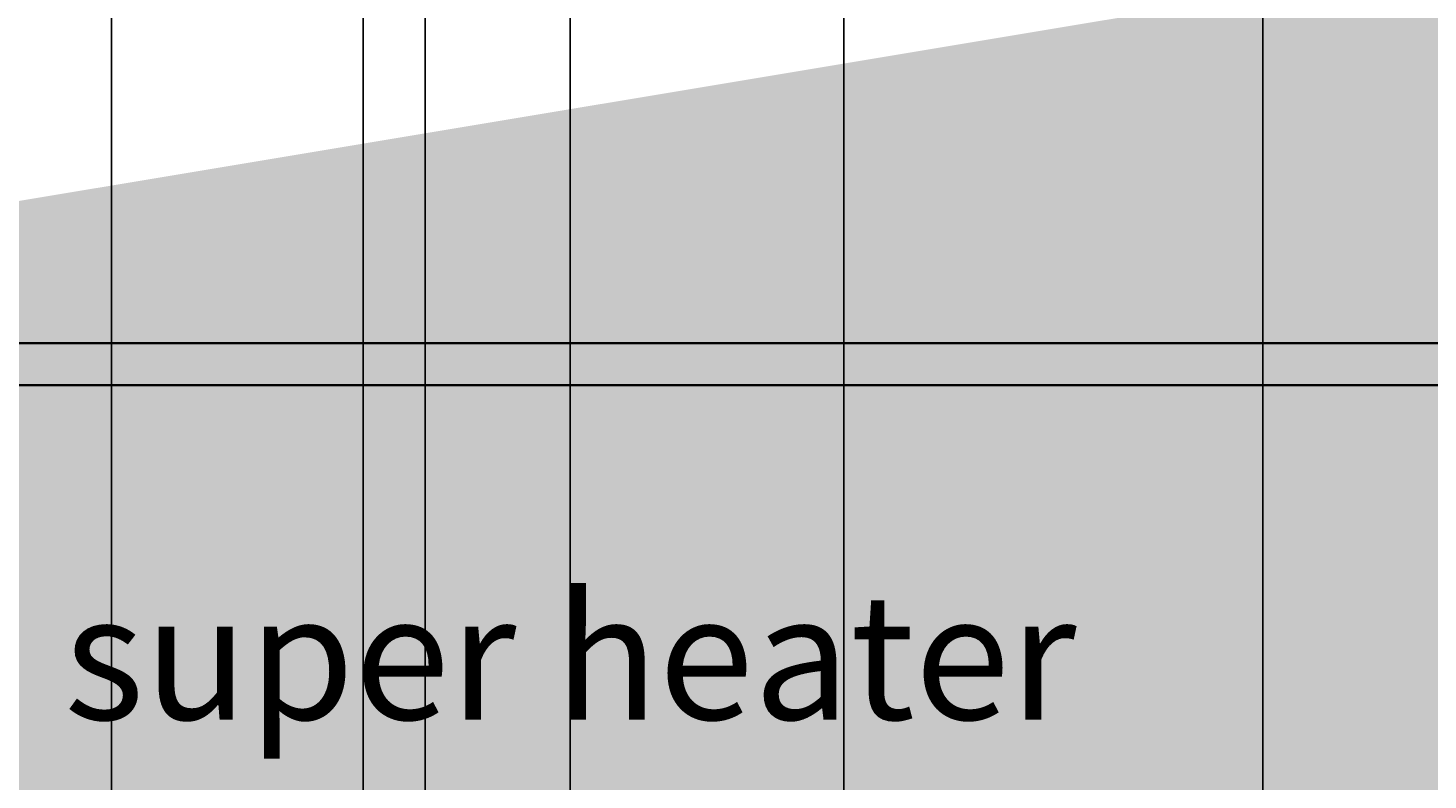
# Model space of a CAD drawing. Units: millimetres. Extents: x -22994 to 29398, y -19990 to 20176.
# Tile 45 of 135: x 136 to 170, y 78 to 96. Entities that reach past the tile are written whole.
import ezdxf

# ---------------------------------------------------------------- set-up
doc = ezdxf.new("R2010")
doc.units = ezdxf.units.MM
doc.header["$MEASUREMENT"] = 0
for name, color, linetype, lineweight in [('M-ANNO-TEXT', 7, 'Continuous', 25), ('M-DIMS', 2, 'Continuous', 18), ('M-EQPM-PATT', 7, 'Continuous', 18), ('M-PIPE', 7, 'Continuous', 35)]:
    doc.layers.add(name, color=color, linetype=linetype, lineweight=lineweight)
doc.styles.get("Standard").update_dxf_attribs({"font": 'arial.ttf'})
doc.dimstyles.get("Standard").update_dxf_attribs({"dimtxt": 0.18, "dimasz": 10000, "dimexe": 0.18, "dimexo": 0.0625, "dimgap": 0.09, "dimtad": 0, "dimtih": 1, "dimtoh": 1, "dimdec": 0, "dimzin": 0, "dimdsep": 46, "dimtxsty": 'Standard', "dimcen": 0.09, "dimadec": 0, "dimazin": 0, "dimtfac": 1, "dimtdec": 0, "dimtofl": 0, "dimtmove": 0, "dimatfit": 3, "dimfxl": 1, "dimtolj": 1, "dimtzin": 0, "dimlwd": 30, "dimarcsym": 0})

# ---------------------------------------------------------------- blocks, each defined once
blk = doc.blocks.new('*D2')
at = {"layer": 'Defpoints', "color": 0, "transparency": 16777216}
for p in [(6.677, 10.271), (290.852, 10.271), (290.852, -5.079)]:
    blk.add_point(p, dxfattribs=at)
at = {"layer": 'M-DIMS', "color": 0, "lineweight": -2, "transparency": 16777216}
for p, q in [((6.677, 10.209), (6.677, -5.259)), ((290.852, 10.209), (290.852, -5.259))]:
    blk.add_line(p, q, dxfattribs=at)
at = {"layer": 'M-DIMS', "color": 0, "lineweight": 30, "transparency": 16777216}
for p, q in [((-9993.323, -5.079), (-19993.323, -5.079)), ((10290.852, -5.079), (20290.852, -5.079))]:
    blk.add_line(p, q, dxfattribs=at)
at = {"layer": 'M-DIMS', "color": 0, "transparency": 16777216}
for points in [[(-9993.323, 1661.588), (-9993.323, -1671.745), (6.677, -5.079)], [(10290.852, 1661.588), (10290.852, -1671.745), (290.852, -5.079)]]:
    blk.add_solid(points, dxfattribs=at)
at = {"layer": 'M-DIMS', "color": 0, "transparency": 16777216, "insert": (148.765, -5.079), "char_height": 0.18, "attachment_point": 5}
blk.add_mtext('\\A1;284.2', dxfattribs=at)
blk = doc.blocks.new('*D3')
at = {"layer": 'Defpoints', "color": 0, "transparency": 16777216}
for p in [(110.265, 204.165), (110.265, 176.366), (95.833, 127.967)]:
    blk.add_point(p, dxfattribs=at)
at = {"layer": 'M-DIMS', "color": 0, "lineweight": -2, "transparency": 16777216}
for p, q in [((95.833, 128.03), (95.833, 204.345)), ((110.265, 176.429), (110.265, 204.345))]:
    blk.add_line(p, q, dxfattribs=at)
at = {"layer": 'M-DIMS', "color": 0, "lineweight": 30, "transparency": 16777216}
for p, q in [((-9904.167, 204.165), (-19904.167, 204.165)), ((10110.265, 204.165), (20110.265, 204.165))]:
    blk.add_line(p, q, dxfattribs=at)
at = {"layer": 'M-DIMS', "color": 0, "transparency": 16777216}
for points in [[(-9904.167, 1870.832), (-9904.167, -1462.501), (95.833, 204.165)], [(10110.265, 1870.832), (10110.265, -1462.501), (110.265, 204.165)]]:
    blk.add_solid(points, dxfattribs=at)
at = {"layer": 'M-DIMS', "color": 0, "transparency": 16777216, "insert": (103.049, 204.165), "char_height": 0.18, "attachment_point": 5}
blk.add_mtext('\\A1;14.432', dxfattribs=at)
blk = doc.blocks.new('*D4')
at = {"layer": 'Defpoints', "color": 0, "transparency": 16777216}
for p in [(116.265, 204.165), (110.265, 176.366), (116.265, 176.366)]:
    blk.add_point(p, dxfattribs=at)
at = {"layer": 'M-DIMS', "color": 0, "lineweight": -2, "transparency": 16777216}
for p, q in [((110.265, 176.429), (110.265, 204.345)), ((116.265, 176.429), (116.265, 204.345))]:
    blk.add_line(p, q, dxfattribs=at)
at = {"layer": 'M-DIMS', "color": 0, "lineweight": 30, "transparency": 16777216}
for p, q in [((-9889.735, 204.165), (-19889.735, 204.165)), ((10116.265, 204.165), (20116.265, 204.165))]:
    blk.add_line(p, q, dxfattribs=at)
at = {"layer": 'M-DIMS', "color": 0, "transparency": 16777216}
for points in [[(-9889.735, 1870.832), (-9889.735, -1462.501), (110.265, 204.165)], [(10116.265, 1870.832), (10116.265, -1462.501), (116.265, 204.165)]]:
    blk.add_solid(points, dxfattribs=at)
at = {"layer": 'M-DIMS', "color": 0, "transparency": 16777216, "insert": (113.265, 204.165), "char_height": 0.18, "attachment_point": 5}
blk.add_mtext('\\A1;6', dxfattribs=at)
blk = doc.blocks.new('*D5')
at = {"layer": 'Defpoints', "color": 0, "transparency": 16777216}
for p in [(181.265, 204.165), (116.265, 176.366), (181.265, 176.366)]:
    blk.add_point(p, dxfattribs=at)
at = {"layer": 'M-DIMS', "color": 0, "lineweight": -2, "transparency": 16777216}
for p, q in [((116.265, 176.429), (116.265, 204.345)), ((181.265, 176.429), (181.265, 204.345))]:
    blk.add_line(p, q, dxfattribs=at)
at = {"layer": 'M-DIMS', "color": 0, "lineweight": 30, "transparency": 16777216}
for p, q in [((-9883.735, 204.165), (-19883.735, 204.165)), ((10181.265, 204.165), (20181.265, 204.165))]:
    blk.add_line(p, q, dxfattribs=at)
at = {"layer": 'M-DIMS', "color": 0, "transparency": 16777216}
for points in [[(-9883.735, 1870.832), (-9883.735, -1462.501), (116.265, 204.165)], [(10181.265, 1870.832), (10181.265, -1462.501), (181.265, 204.165)]]:
    blk.add_solid(points, dxfattribs=at)
at = {"layer": 'M-DIMS', "color": 0, "transparency": 16777216, "insert": (148.765, 204.165), "char_height": 0.18, "attachment_point": 5}
blk.add_mtext('\\A1;65', dxfattribs=at)
blk = doc.blocks.new('*D6')
at = {"layer": 'Defpoints', "color": 0, "transparency": 16777216}
for p in [(187.265, 204.165), (181.265, 176.366), (187.265, 176.366)]:
    blk.add_point(p, dxfattribs=at)
at = {"layer": 'M-DIMS', "color": 0, "lineweight": -2, "transparency": 16777216}
for p, q in [((181.265, 176.429), (181.265, 204.345)), ((187.265, 176.429), (187.265, 204.345))]:
    blk.add_line(p, q, dxfattribs=at)
at = {"layer": 'M-DIMS', "color": 0, "lineweight": 30, "transparency": 16777216}
for p, q in [((-9818.735, 204.165), (-19818.735, 204.165)), ((10187.265, 204.165), (20187.265, 204.165))]:
    blk.add_line(p, q, dxfattribs=at)
at = {"layer": 'M-DIMS', "color": 0, "transparency": 16777216}
for points in [[(-9818.735, 1870.832), (-9818.735, -1462.501), (181.265, 204.165)], [(10187.265, 1870.832), (10187.265, -1462.501), (187.265, 204.165)]]:
    blk.add_solid(points, dxfattribs=at)
at = {"layer": 'M-DIMS', "color": 0, "transparency": 16777216, "insert": (184.265, 204.165), "char_height": 0.18, "attachment_point": 5}
blk.add_mtext('\\A1;6', dxfattribs=at)
blk = doc.blocks.new('*D7')
at = {"layer": 'Defpoints', "color": 0, "transparency": 16777216}
for p in [(201.697, 204.165), (187.265, 176.366), (201.697, 127.967)]:
    blk.add_point(p, dxfattribs=at)
at = {"layer": 'M-DIMS', "color": 0, "lineweight": -2, "transparency": 16777216}
for p, q in [((187.265, 176.429), (187.265, 204.345)), ((201.697, 128.03), (201.697, 204.345))]:
    blk.add_line(p, q, dxfattribs=at)
at = {"layer": 'M-DIMS', "color": 0, "lineweight": 30, "transparency": 16777216}
for p, q in [((-9812.735, 204.165), (-19812.735, 204.165)), ((10201.697, 204.165), (20201.697, 204.165))]:
    blk.add_line(p, q, dxfattribs=at)
at = {"layer": 'M-DIMS', "color": 0, "transparency": 16777216}
for points in [[(-9812.735, 1870.832), (-9812.735, -1462.501), (187.265, 204.165)], [(10201.697, 1870.832), (10201.697, -1462.501), (201.697, 204.165)]]:
    blk.add_solid(points, dxfattribs=at)
at = {"layer": 'M-DIMS', "color": 0, "transparency": 16777216, "insert": (194.481, 204.165), "char_height": 0.18, "attachment_point": 5}
blk.add_mtext('\\A1;14.432', dxfattribs=at)
blk = doc.blocks.new('*D8')
at = {"layer": 'Defpoints', "color": 0, "transparency": 16777216}
for p in [(227.648, 204.165), (227.648, 146.73), (201.697, 127.967)]:
    blk.add_point(p, dxfattribs=at)
at = {"layer": 'M-DIMS', "color": 0, "lineweight": -2, "transparency": 16777216}
for p, q in [((201.697, 128.03), (201.697, 204.345)), ((227.648, 146.792), (227.648, 204.345))]:
    blk.add_line(p, q, dxfattribs=at)
at = {"layer": 'M-DIMS', "color": 0, "lineweight": 30, "transparency": 16777216}
for p, q in [((-9798.303, 204.165), (-19798.303, 204.165)), ((10227.648, 204.165), (20227.648, 204.165))]:
    blk.add_line(p, q, dxfattribs=at)
at = {"layer": 'M-DIMS', "color": 0, "transparency": 16777216}
for points in [[(-9798.303, 1870.832), (-9798.303, -1462.501), (201.697, 204.165)], [(10227.648, 1870.832), (10227.648, -1462.501), (227.648, 204.165)]]:
    blk.add_solid(points, dxfattribs=at)
at = {"layer": 'M-DIMS', "color": 0, "transparency": 16777216, "insert": (214.673, 204.165), "char_height": 0.18, "attachment_point": 5}
blk.add_mtext('\\A1;25.95', dxfattribs=at)
blk = doc.blocks.new('*D9')
at = {"layer": 'Defpoints', "color": 0, "transparency": 16777216}
for p in [(187.265, 176.366), (306.202, 176.366), (290.852, 10.271)]:
    blk.add_point(p, dxfattribs=at)
at = {"layer": 'M-DIMS', "color": 0, "lineweight": 30, "transparency": 16777216}
for p, q in [((306.202, 10176.366), (306.202, 20176.366)), ((306.202, -9989.729), (306.202, -19989.729))]:
    blk.add_line(p, q, dxfattribs=at)
at = {"layer": 'M-DIMS', "color": 0, "lineweight": -2, "transparency": 16777216}
for p, q in [((187.327, 176.366), (306.382, 176.366)), ((290.915, 10.271), (306.382, 10.271))]:
    blk.add_line(p, q, dxfattribs=at)
at = {"layer": 'M-DIMS', "color": 0, "transparency": 16777216}
for points in [[(-1360.465, 10176.366), (1972.869, 10176.366), (306.202, 176.366)], [(-1360.465, -9989.729), (1972.869, -9989.729), (306.202, 10.271)]]:
    blk.add_solid(points, dxfattribs=at)
at = {"layer": 'M-DIMS', "color": 0, "transparency": 16777216, "insert": (306.202, 93.319), "char_height": 0.18, "attachment_point": 5}
blk.add_mtext('\\A1;166.1', dxfattribs=at)
blk = doc.blocks.new('*D10')
at = {"layer": 'Defpoints', "color": 0, "transparency": 16777216}
for p in [(125.65, 136.071), (133.346, 136.071), (133.346, -5.079)]:
    blk.add_point(p, dxfattribs=at)
at = {"layer": 'M-DIMS', "color": 0, "lineweight": -2, "transparency": 16777216}
for p, q in [((125.65, 136.009), (125.65, -5.259)), ((133.346, 136.009), (133.346, -5.259))]:
    blk.add_line(p, q, dxfattribs=at)
at = {"layer": 'M-DIMS', "color": 0, "lineweight": 30, "transparency": 16777216}
for p, q in [((-9874.35, -5.079), (-19874.35, -5.079)), ((10133.346, -5.079), (20133.346, -5.079))]:
    blk.add_line(p, q, dxfattribs=at)
at = {"layer": 'M-DIMS', "color": 0, "transparency": 16777216}
for points in [[(-9874.35, 1661.588), (-9874.35, -1671.745), (125.65, -5.079)], [(10133.346, 1661.588), (10133.346, -1671.745), (133.346, -5.079)]]:
    blk.add_solid(points, dxfattribs=at)
at = {"layer": 'M-DIMS', "color": 0, "transparency": 16777216, "insert": (129.498, -5.079), "char_height": 0.18, "attachment_point": 5}
blk.add_mtext('\\A1;7.696', dxfattribs=at)
blk = doc.blocks.new('*D11')
at = {"layer": 'Defpoints', "color": 0, "transparency": 16777216}
for p in [(133.346, 136.071), (135.65, 136.071), (135.65, -5.079)]:
    blk.add_point(p, dxfattribs=at)
at = {"layer": 'M-DIMS', "color": 0, "lineweight": -2, "transparency": 16777216}
for p, q in [((133.346, 136.009), (133.346, -5.259)), ((135.65, 136.009), (135.65, -5.259))]:
    blk.add_line(p, q, dxfattribs=at)
at = {"layer": 'M-DIMS', "color": 0, "lineweight": 30, "transparency": 16777216}
for p, q in [((-9866.654, -5.079), (-19866.654, -5.079)), ((10135.65, -5.079), (20135.65, -5.079))]:
    blk.add_line(p, q, dxfattribs=at)
at = {"layer": 'M-DIMS', "color": 0, "transparency": 16777216}
for points in [[(-9866.654, 1661.588), (-9866.654, -1671.745), (133.346, -5.079)], [(10135.65, 1661.588), (10135.65, -1671.745), (135.65, -5.079)]]:
    blk.add_solid(points, dxfattribs=at)
at = {"layer": 'M-DIMS', "color": 0, "transparency": 16777216, "insert": (134.498, -5.079), "char_height": 0.18, "attachment_point": 5}
blk.add_mtext('\\A1;2.304', dxfattribs=at)
blk = doc.blocks.new('*D12')
at = {"layer": 'Defpoints', "color": 0, "transparency": 16777216}
for p in [(135.65, 136.071), (145.65, 136.071), (145.65, -5.079)]:
    blk.add_point(p, dxfattribs=at)
at = {"layer": 'M-DIMS', "color": 0, "lineweight": -2, "transparency": 16777216}
for p, q in [((135.65, 136.009), (135.65, -5.259)), ((145.65, 136.009), (145.65, -5.259))]:
    blk.add_line(p, q, dxfattribs=at)
at = {"layer": 'M-DIMS', "color": 0, "lineweight": 30, "transparency": 16777216}
for p, q in [((-9864.35, -5.079), (-19864.35, -5.079)), ((10145.65, -5.079), (20145.65, -5.079))]:
    blk.add_line(p, q, dxfattribs=at)
at = {"layer": 'M-DIMS', "color": 0, "transparency": 16777216}
for points in [[(-9864.35, 1661.588), (-9864.35, -1671.745), (135.65, -5.079)], [(10145.65, 1661.588), (10145.65, -1671.745), (145.65, -5.079)]]:
    blk.add_solid(points, dxfattribs=at)
at = {"layer": 'M-DIMS', "color": 0, "transparency": 16777216, "insert": (140.65, -5.079), "char_height": 0.18, "attachment_point": 5}
blk.add_mtext('\\A1;10', dxfattribs=at)
blk = doc.blocks.new('*D13')
at = {"layer": 'Defpoints', "color": 0, "transparency": 16777216}
for p in [(145.65, 136.071), (155.65, 136.071), (155.65, -5.079)]:
    blk.add_point(p, dxfattribs=at)
at = {"layer": 'M-DIMS', "color": 0, "lineweight": -2, "transparency": 16777216}
for p, q in [((145.65, 136.009), (145.65, -5.259)), ((155.65, 136.009), (155.65, -5.259))]:
    blk.add_line(p, q, dxfattribs=at)
at = {"layer": 'M-DIMS', "color": 0, "lineweight": 30, "transparency": 16777216}
for p, q in [((-9854.35, -5.079), (-19854.35, -5.079)), ((10155.65, -5.079), (20155.65, -5.079))]:
    blk.add_line(p, q, dxfattribs=at)
at = {"layer": 'M-DIMS', "color": 0, "transparency": 16777216}
for points in [[(-9854.35, 1661.588), (-9854.35, -1671.745), (145.65, -5.079)], [(10155.65, 1661.588), (10155.65, -1671.745), (155.65, -5.079)]]:
    blk.add_solid(points, dxfattribs=at)
at = {"layer": 'M-DIMS', "color": 0, "transparency": 16777216, "insert": (150.65, -5.079), "char_height": 0.18, "attachment_point": 5}
blk.add_mtext('\\A1;10', dxfattribs=at)
blk = doc.blocks.new('*D14')
at = {"layer": 'Defpoints', "color": 0, "transparency": 16777216}
for p in [(155.65, 136.071), (165.65, 136.071), (165.65, -5.079)]:
    blk.add_point(p, dxfattribs=at)
at = {"layer": 'M-DIMS', "color": 0, "lineweight": -2, "transparency": 16777216}
for p, q in [((155.65, 136.009), (155.65, -5.259)), ((165.65, 136.009), (165.65, -5.259))]:
    blk.add_line(p, q, dxfattribs=at)
at = {"layer": 'M-DIMS', "color": 0, "lineweight": 30, "transparency": 16777216}
for p, q in [((-9844.35, -5.079), (-19844.35, -5.079)), ((10165.65, -5.079), (20165.65, -5.079))]:
    blk.add_line(p, q, dxfattribs=at)
at = {"layer": 'M-DIMS', "color": 0, "transparency": 16777216}
for points in [[(-9844.35, 1661.588), (-9844.35, -1671.745), (155.65, -5.079)], [(10165.65, 1661.588), (10165.65, -1671.745), (165.65, -5.079)]]:
    blk.add_solid(points, dxfattribs=at)
at = {"layer": 'M-DIMS', "color": 0, "transparency": 16777216, "insert": (160.65, -5.079), "char_height": 0.18, "attachment_point": 5}
blk.add_mtext('\\A1;10', dxfattribs=at)
blk = doc.blocks.new('*D15')
at = {"layer": 'Defpoints', "color": 0, "transparency": 16777216}
for p in [(173.346, 154.788), (173.346, 136.071), (306.202, 136.071)]:
    blk.add_point(p, dxfattribs=at)
at = {"layer": 'M-DIMS', "color": 0, "lineweight": 30, "transparency": 16777216}
for p, q in [((306.202, 10154.788), (306.202, 20154.788)), ((306.202, -9863.929), (306.202, -19863.929))]:
    blk.add_line(p, q, dxfattribs=at)
at = {"layer": 'M-DIMS', "color": 0, "lineweight": -2, "transparency": 16777216}
for p, q in [((173.408, 154.788), (306.382, 154.788)), ((173.408, 136.071), (306.382, 136.071))]:
    blk.add_line(p, q, dxfattribs=at)
at = {"layer": 'M-DIMS', "color": 0, "transparency": 16777216}
for points in [[(-1360.465, 10154.788), (1972.869, 10154.788), (306.202, 154.788)], [(-1360.465, -9863.929), (1972.869, -9863.929), (306.202, 136.071)]]:
    blk.add_solid(points, dxfattribs=at)
at = {"layer": 'M-DIMS', "color": 0, "transparency": 16777216, "insert": (306.202, 145.43), "char_height": 0.18, "attachment_point": 5}
blk.add_mtext('\\A1;18.717', dxfattribs=at)
blk = doc.blocks.new('*D16')
at = {"layer": 'Defpoints', "color": 0, "transparency": 16777216}
for p in [(120.17, 204.165), (110.466, 48.035), (120.17, 48.035)]:
    blk.add_point(p, dxfattribs=at)
at = {"layer": 'M-DIMS', "color": 0, "lineweight": -2, "transparency": 16777216}
for p, q in [((110.466, 48.097), (110.466, 204.345)), ((120.17, 48.097), (120.17, 204.345))]:
    blk.add_line(p, q, dxfattribs=at)
at = {"layer": 'M-DIMS', "color": 0, "lineweight": 30, "transparency": 16777216}
for p, q in [((-9889.534, 204.165), (-19889.534, 204.165)), ((10120.17, 204.165), (20120.17, 204.165))]:
    blk.add_line(p, q, dxfattribs=at)
at = {"layer": 'M-DIMS', "color": 0, "transparency": 16777216}
for points in [[(-9889.534, 1870.832), (-9889.534, -1462.501), (110.466, 204.165)], [(10120.17, 1870.832), (10120.17, -1462.501), (120.17, 204.165)]]:
    blk.add_solid(points, dxfattribs=at)
at = {"layer": 'M-DIMS', "color": 0, "transparency": 16777216, "insert": (115.318, 204.165), "char_height": 0.18, "attachment_point": 5}
blk.add_mtext('\\A1;9.704', dxfattribs=at)
blk = doc.blocks.new('*D17')
at = {"layer": 'Defpoints', "color": 0, "transparency": 16777216}
for p in [(126.17, 204.165), (120.17, 48.035), (126.17, 48.035)]:
    blk.add_point(p, dxfattribs=at)
at = {"layer": 'M-DIMS', "color": 0, "lineweight": -2, "transparency": 16777216}
for p, q in [((120.17, 48.097), (120.17, 204.345)), ((126.17, 48.097), (126.17, 204.345))]:
    blk.add_line(p, q, dxfattribs=at)
at = {"layer": 'M-DIMS', "color": 0, "lineweight": 30, "transparency": 16777216}
for p, q in [((-9879.83, 204.165), (-19879.83, 204.165)), ((10126.17, 204.165), (20126.17, 204.165))]:
    blk.add_line(p, q, dxfattribs=at)
at = {"layer": 'M-DIMS', "color": 0, "transparency": 16777216}
for points in [[(-9879.83, 1870.832), (-9879.83, -1462.501), (120.17, 204.165)], [(10126.17, 1870.832), (10126.17, -1462.501), (126.17, 204.165)]]:
    blk.add_solid(points, dxfattribs=at)
at = {"layer": 'M-DIMS', "color": 0, "transparency": 16777216, "insert": (123.17, 204.165), "char_height": 0.18, "attachment_point": 5}
blk.add_mtext('\\A1;6', dxfattribs=at)
blk = doc.blocks.new('*D18')
at = {"layer": 'Defpoints', "color": 0, "transparency": 16777216}
for p in [(132.17, 204.165), (126.17, 48.035), (132.17, 48.035)]:
    blk.add_point(p, dxfattribs=at)
at = {"layer": 'M-DIMS', "color": 0, "lineweight": -2, "transparency": 16777216}
for p, q in [((126.17, 48.097), (126.17, 204.345)), ((132.17, 48.097), (132.17, 204.345))]:
    blk.add_line(p, q, dxfattribs=at)
at = {"layer": 'M-DIMS', "color": 0, "lineweight": 30, "transparency": 16777216}
for p, q in [((-9873.83, 204.165), (-19873.83, 204.165)), ((10132.17, 204.165), (20132.17, 204.165))]:
    blk.add_line(p, q, dxfattribs=at)
at = {"layer": 'M-DIMS', "color": 0, "transparency": 16777216}
for points in [[(-9873.83, 1870.832), (-9873.83, -1462.501), (126.17, 204.165)], [(10132.17, 1870.832), (10132.17, -1462.501), (132.17, 204.165)]]:
    blk.add_solid(points, dxfattribs=at)
at = {"layer": 'M-DIMS', "color": 0, "transparency": 16777216, "insert": (129.17, 204.165), "char_height": 0.18, "attachment_point": 5}
blk.add_mtext('\\A1;6', dxfattribs=at)
blk = doc.blocks.new('*D19')
at = {"layer": 'Defpoints', "color": 0, "transparency": 16777216}
for p in [(138.17, 204.165), (132.17, 48.035), (138.17, 48.035)]:
    blk.add_point(p, dxfattribs=at)
at = {"layer": 'M-DIMS', "color": 0, "lineweight": -2, "transparency": 16777216}
for p, q in [((132.17, 48.097), (132.17, 204.345)), ((138.17, 48.097), (138.17, 204.345))]:
    blk.add_line(p, q, dxfattribs=at)
at = {"layer": 'M-DIMS', "color": 0, "lineweight": 30, "transparency": 16777216}
for p, q in [((-9867.83, 204.165), (-19867.83, 204.165)), ((10138.17, 204.165), (20138.17, 204.165))]:
    blk.add_line(p, q, dxfattribs=at)
at = {"layer": 'M-DIMS', "color": 0, "transparency": 16777216}
for points in [[(-9867.83, 1870.832), (-9867.83, -1462.501), (132.17, 204.165)], [(10138.17, 1870.832), (10138.17, -1462.501), (138.17, 204.165)]]:
    blk.add_solid(points, dxfattribs=at)
at = {"layer": 'M-DIMS', "color": 0, "transparency": 16777216, "insert": (135.17, 204.165), "char_height": 0.18, "attachment_point": 5}
blk.add_mtext('\\A1;6', dxfattribs=at)
blk = doc.blocks.new('*D20')
at = {"layer": 'Defpoints', "color": 0, "transparency": 16777216}
for p in [(144.17, 204.165), (138.17, 48.035), (144.17, 48.035)]:
    blk.add_point(p, dxfattribs=at)
at = {"layer": 'M-DIMS', "color": 0, "lineweight": -2, "transparency": 16777216}
for p, q in [((138.17, 48.097), (138.17, 204.345)), ((144.17, 48.097), (144.17, 204.345))]:
    blk.add_line(p, q, dxfattribs=at)
at = {"layer": 'M-DIMS', "color": 0, "lineweight": 30, "transparency": 16777216}
for p, q in [((-9861.83, 204.165), (-19861.83, 204.165)), ((10144.17, 204.165), (20144.17, 204.165))]:
    blk.add_line(p, q, dxfattribs=at)
at = {"layer": 'M-DIMS', "color": 0, "transparency": 16777216}
for points in [[(-9861.83, 1870.832), (-9861.83, -1462.501), (138.17, 204.165)], [(10144.17, 1870.832), (10144.17, -1462.501), (144.17, 204.165)]]:
    blk.add_solid(points, dxfattribs=at)
at = {"layer": 'M-DIMS', "color": 0, "transparency": 16777216, "insert": (141.17, 204.165), "char_height": 0.18, "attachment_point": 5}
blk.add_mtext('\\A1;6', dxfattribs=at)
blk = doc.blocks.new('*D21')
at = {"layer": 'Defpoints', "color": 0, "transparency": 16777216}
for p in [(149.116, 204.165), (144.17, 48.035), (149.116, 48.035)]:
    blk.add_point(p, dxfattribs=at)
at = {"layer": 'M-DIMS', "color": 0, "lineweight": -2, "transparency": 16777216}
for p, q in [((144.17, 48.097), (144.17, 204.345)), ((149.116, 48.097), (149.116, 204.345))]:
    blk.add_line(p, q, dxfattribs=at)
at = {"layer": 'M-DIMS', "color": 0, "lineweight": 30, "transparency": 16777216}
for p, q in [((-9855.83, 204.165), (-19855.83, 204.165)), ((10149.116, 204.165), (20149.116, 204.165))]:
    blk.add_line(p, q, dxfattribs=at)
at = {"layer": 'M-DIMS', "color": 0, "transparency": 16777216}
for points in [[(-9855.83, 1870.832), (-9855.83, -1462.501), (144.17, 204.165)], [(10149.116, 1870.832), (10149.116, -1462.501), (149.116, 204.165)]]:
    blk.add_solid(points, dxfattribs=at)
at = {"layer": 'M-DIMS', "color": 0, "transparency": 16777216, "insert": (146.643, 204.165), "char_height": 0.18, "attachment_point": 5}
blk.add_mtext('\\A1;4.945', dxfattribs=at)
blk = doc.blocks.new('*D22')
at = {"layer": 'Defpoints', "color": 0, "transparency": 16777216}
for p in [(149.116, 30.99), (155.116, 30.99), (155.116, -5.079)]:
    blk.add_point(p, dxfattribs=at)
at = {"layer": 'M-DIMS', "color": 0, "lineweight": -2, "transparency": 16777216}
for p, q in [((149.116, 30.927), (149.116, -5.259)), ((155.116, 30.927), (155.116, -5.259))]:
    blk.add_line(p, q, dxfattribs=at)
at = {"layer": 'M-DIMS', "color": 0, "lineweight": 30, "transparency": 16777216}
for p, q in [((-9850.884, -5.079), (-19850.884, -5.079)), ((10155.116, -5.079), (20155.116, -5.079))]:
    blk.add_line(p, q, dxfattribs=at)
at = {"layer": 'M-DIMS', "color": 0, "transparency": 16777216}
for points in [[(-9850.884, 1661.588), (-9850.884, -1671.745), (149.116, -5.079)], [(10155.116, 1661.588), (10155.116, -1671.745), (155.116, -5.079)]]:
    blk.add_solid(points, dxfattribs=at)
at = {"layer": 'M-DIMS', "color": 0, "transparency": 16777216, "insert": (152.116, -5.079), "char_height": 0.18, "attachment_point": 5}
blk.add_mtext('\\A1;6', dxfattribs=at)
blk = doc.blocks.new('*D23')
at = {"layer": 'Defpoints', "color": 0, "transparency": 16777216}
for p in [(155.116, 30.99), (161.116, 30.99), (161.116, -5.079)]:
    blk.add_point(p, dxfattribs=at)
at = {"layer": 'M-DIMS', "color": 0, "lineweight": -2, "transparency": 16777216}
for p, q in [((155.116, 30.927), (155.116, -5.259)), ((161.116, 30.927), (161.116, -5.259))]:
    blk.add_line(p, q, dxfattribs=at)
at = {"layer": 'M-DIMS', "color": 0, "lineweight": 30, "transparency": 16777216}
for p, q in [((-9844.884, -5.079), (-19844.884, -5.079)), ((10161.116, -5.079), (20161.116, -5.079))]:
    blk.add_line(p, q, dxfattribs=at)
at = {"layer": 'M-DIMS', "color": 0, "transparency": 16777216}
for points in [[(-9844.884, 1661.588), (-9844.884, -1671.745), (155.116, -5.079)], [(10161.116, 1661.588), (10161.116, -1671.745), (161.116, -5.079)]]:
    blk.add_solid(points, dxfattribs=at)
at = {"layer": 'M-DIMS', "color": 0, "transparency": 16777216, "insert": (158.116, -5.079), "char_height": 0.18, "attachment_point": 5}
blk.add_mtext('\\A1;6', dxfattribs=at)
blk = doc.blocks.new('*D24')
at = {"layer": 'Defpoints', "color": 0, "transparency": 16777216}
for p in [(161.116, 30.99), (166.439, 30.99), (166.439, -5.079)]:
    blk.add_point(p, dxfattribs=at)
at = {"layer": 'M-DIMS', "color": 0, "lineweight": -2, "transparency": 16777216}
for p, q in [((161.116, 30.927), (161.116, -5.259)), ((166.439, 30.927), (166.439, -5.259))]:
    blk.add_line(p, q, dxfattribs=at)
at = {"layer": 'M-DIMS', "color": 0, "lineweight": 30, "transparency": 16777216}
for p, q in [((-9838.884, -5.079), (-19838.884, -5.079)), ((10166.439, -5.079), (20166.439, -5.079))]:
    blk.add_line(p, q, dxfattribs=at)
at = {"layer": 'M-DIMS', "color": 0, "transparency": 16777216}
for points in [[(-9838.884, 1661.588), (-9838.884, -1671.745), (161.116, -5.079)], [(10166.439, 1661.588), (10166.439, -1671.745), (166.439, -5.079)]]:
    blk.add_solid(points, dxfattribs=at)
at = {"layer": 'M-DIMS', "color": 0, "transparency": 16777216, "insert": (163.777, -5.079), "char_height": 0.18, "attachment_point": 5}
blk.add_mtext('\\A1;5.323', dxfattribs=at)
blk = doc.blocks.new('*D25')
at = {"layer": 'Defpoints', "color": 0, "transparency": 16777216}
for p in [(166.439, 30.99), (172.439, 30.99), (172.439, -5.079)]:
    blk.add_point(p, dxfattribs=at)
at = {"layer": 'M-DIMS', "color": 0, "lineweight": -2, "transparency": 16777216}
for p, q in [((166.439, 30.927), (166.439, -5.259)), ((172.439, 30.927), (172.439, -5.259))]:
    blk.add_line(p, q, dxfattribs=at)
at = {"layer": 'M-DIMS', "color": 0, "lineweight": 30, "transparency": 16777216}
for p, q in [((-9833.561, -5.079), (-19833.561, -5.079)), ((10172.439, -5.079), (20172.439, -5.079))]:
    blk.add_line(p, q, dxfattribs=at)
at = {"layer": 'M-DIMS', "color": 0, "transparency": 16777216}
for points in [[(-9833.561, 1661.588), (-9833.561, -1671.745), (166.439, -5.079)], [(10172.439, 1661.588), (10172.439, -1671.745), (172.439, -5.079)]]:
    blk.add_solid(points, dxfattribs=at)
at = {"layer": 'M-DIMS', "color": 0, "transparency": 16777216, "insert": (169.439, -5.079), "char_height": 0.18, "attachment_point": 5}
blk.add_mtext('\\A1;6', dxfattribs=at)
blk = doc.blocks.new('*D26')
at = {"layer": 'Defpoints', "color": 0, "transparency": 16777216}
for p in [(172.439, 30.99), (178.439, 30.99), (178.439, -5.079)]:
    blk.add_point(p, dxfattribs=at)
at = {"layer": 'M-DIMS', "color": 0, "lineweight": -2, "transparency": 16777216}
for p, q in [((172.439, 30.927), (172.439, -5.259)), ((178.439, 30.927), (178.439, -5.259))]:
    blk.add_line(p, q, dxfattribs=at)
at = {"layer": 'M-DIMS', "color": 0, "lineweight": 30, "transparency": 16777216}
for p, q in [((-9827.561, -5.079), (-19827.561, -5.079)), ((10178.439, -5.079), (20178.439, -5.079))]:
    blk.add_line(p, q, dxfattribs=at)
at = {"layer": 'M-DIMS', "color": 0, "transparency": 16777216}
for points in [[(-9827.561, 1661.588), (-9827.561, -1671.745), (172.439, -5.079)], [(10178.439, 1661.588), (10178.439, -1671.745), (178.439, -5.079)]]:
    blk.add_solid(points, dxfattribs=at)
at = {"layer": 'M-DIMS', "color": 0, "transparency": 16777216, "insert": (175.439, -5.079), "char_height": 0.18, "attachment_point": 5}
blk.add_mtext('\\A1;6', dxfattribs=at)
blk = doc.blocks.new('*D27')
at = {"layer": 'Defpoints', "color": 0, "transparency": 16777216}
for p in [(178.439, 30.99), (188.117, 30.99), (188.117, -5.079)]:
    blk.add_point(p, dxfattribs=at)
at = {"layer": 'M-DIMS', "color": 0, "lineweight": -2, "transparency": 16777216}
for p, q in [((178.439, 30.927), (178.439, -5.259)), ((188.117, 30.927), (188.117, -5.259))]:
    blk.add_line(p, q, dxfattribs=at)
at = {"layer": 'M-DIMS', "color": 0, "lineweight": 30, "transparency": 16777216}
for p, q in [((-9821.561, -5.079), (-19821.561, -5.079)), ((10188.117, -5.079), (20188.117, -5.079))]:
    blk.add_line(p, q, dxfattribs=at)
at = {"layer": 'M-DIMS', "color": 0, "transparency": 16777216}
for points in [[(-9821.561, 1661.588), (-9821.561, -1671.745), (178.439, -5.079)], [(10188.117, 1661.588), (10188.117, -1671.745), (188.117, -5.079)]]:
    blk.add_solid(points, dxfattribs=at)
at = {"layer": 'M-DIMS', "color": 0, "transparency": 16777216, "insert": (183.278, -5.079), "char_height": 0.18, "attachment_point": 5}
blk.add_mtext('\\A1;9.679', dxfattribs=at)
blk = doc.blocks.new('*D28')
at = {"layer": 'Defpoints', "color": 0, "transparency": 16777216}
for p in [(188.117, 48.035), (306.202, 48.035), (188.117, 30.99)]:
    blk.add_point(p, dxfattribs=at)
at = {"layer": 'M-DIMS', "color": 0, "lineweight": 30, "transparency": 16777216}
for p, q in [((306.202, 10048.035), (306.202, 20048.035)), ((306.202, -9969.01), (306.202, -19969.01))]:
    blk.add_line(p, q, dxfattribs=at)
at = {"layer": 'M-DIMS', "color": 0, "lineweight": -2, "transparency": 16777216}
for p, q in [((188.18, 48.035), (306.382, 48.035)), ((188.18, 30.99), (306.382, 30.99))]:
    blk.add_line(p, q, dxfattribs=at)
at = {"layer": 'M-DIMS', "color": 0, "transparency": 16777216}
for points in [[(-1360.465, 10048.035), (1972.869, 10048.035), (306.202, 48.035)], [(-1360.465, -9969.01), (1972.869, -9969.01), (306.202, 30.99)]]:
    blk.add_solid(points, dxfattribs=at)
at = {"layer": 'M-DIMS', "color": 0, "transparency": 16777216, "insert": (306.202, 39.512), "char_height": 0.18, "attachment_point": 5}
blk.add_mtext('\\A1;17.045', dxfattribs=at)
blk = doc.blocks.new('*D29')
at = {"layer": 'Defpoints', "color": 0, "transparency": 16777216}
for p in [(36.801, 80.045), (64.03, 80.045)]:
    blk.add_point(p, dxfattribs=at)
at = {"layer": 'M-DIMS', "color": 0, "lineweight": -2, "transparency": 16777216}
for p, q in [((50.325, 80.045), (50.505, 80.045)), ((50.415, 79.955), (50.415, 80.135))]:
    blk.add_line(p, q, dxfattribs=at)
at = {"layer": 'M-DIMS', "color": 0, "lineweight": 30, "transparency": 16777216}
blk.add_line((20064.03, 80.03), (10064.03, 80.038), dxfattribs=at)
at = {"layer": 'M-DIMS', "color": 0, "transparency": 16777216}
blk.add_solid([(10064.031, 1746.704), (10064.028, -1586.629), (64.03, 80.045)], dxfattribs=at)
at = {"layer": 'M-DIMS', "color": 0, "transparency": 16777216, "insert": (20064.521, 80.03), "char_height": 0.18, "attachment_point": 5}
blk.add_mtext('\\A1;∅27.23', dxfattribs=at)
blk = doc.blocks.new('*D36')
at = {"layer": 'Defpoints', "color": 0, "transparency": 16777216}
for p in [(46.39, 31.303), (46.387, 26.593)]:
    blk.add_point(p, dxfattribs=at)
at = {"layer": 'M-DIMS', "color": 0, "lineweight": 30, "transparency": 16777216}
for p, q in [((57.15, 20031.301), (51.77, 10031.302)), ((10057.15, 20031.301), (57.15, 20031.301))]:
    blk.add_line(p, q, dxfattribs=at)
at = {"layer": 'M-DIMS', "color": 0, "lineweight": -2, "transparency": 16777216}
for p, q in [((46.299, 28.948), (46.479, 28.948)), ((46.389, 28.858), (46.389, 29.038))]:
    blk.add_line(p, q, dxfattribs=at)
at = {"layer": 'M-DIMS', "color": 0, "transparency": 16777216}
blk.add_solid([(-1614.896, 10032.199), (1718.436, 10030.405), (46.39, 31.303)], dxfattribs=at)
at = {"layer": 'M-DIMS', "color": 0, "transparency": 16777216, "insert": (10057.554, 20031.301), "char_height": 0.18, "attachment_point": 5}
blk.add_mtext('\\A1;∅4.71', dxfattribs=at)
blk = doc.blocks.new('*D37')
at = {"layer": 'Defpoints', "color": 0, "transparency": 16777216}
for p in [(54.834, 118.615), (59.494, 118.614)]:
    blk.add_point(p, dxfattribs=at)
at = {"layer": 'M-DIMS', "color": 0, "lineweight": -2, "transparency": 16777216}
for p, q in [((57.164, 118.524), (57.164, 118.704)), ((57.074, 118.614), (57.254, 118.614))]:
    blk.add_line(p, q, dxfattribs=at)
at = {"layer": 'M-DIMS', "color": 0, "lineweight": 30, "transparency": 16777216}
blk.add_line((20059.493, 116.253), (10059.494, 117.434), dxfattribs=at)
at = {"layer": 'M-DIMS', "color": 0, "transparency": 16777216}
blk.add_solid([(10059.69, 1784.1), (10059.297, -1549.233), (59.494, 118.614)], dxfattribs=at)
at = {"layer": 'M-DIMS', "color": 0, "transparency": 16777216, "insert": (20059.985, 116.253), "char_height": 0.18, "attachment_point": 5}
blk.add_mtext('\\A1;∅4.659', dxfattribs=at)

msp = doc.modelspace()

# ---------------------------------------------------------------- hatches: boundary and pattern name
at = {"layer": 'M-EQPM-PATT'}
h = msp.add_hatch(color=256, dxfattribs=at)
h.set_gradient(color1=(205, 32, 39), color2=(205, 32, 39), tint=1)
h.paths.add_polyline_path([(116.2647, 150.3662), (116.2647, 170.3662), (116.2647, 176.3662), (110.2647, 176.3662), (110.2647, 152.0276), (95.8327, 127.967), (95.8327, 16.6063), (201.6967, 16.6063), (201.6967, 127.967), (187.2647, 152.0276), (187.2647, 176.3662), (181.2647, 176.3662), (181.2647, 170.3662), (181.2647, 150.3662), (195.6967, 126.3055), (195.6967, 22.6063), (101.8327, 22.6063), (101.8327, 126.3055)])
h.paths.add_polyline_path([(185.2208, 88.6347), (101.8327, 88.6347), (101.8327, 87.6347), (182.8066, 87.6347), (178.7313, 83.5594), (195.6967, 83.5594), (195.6967, 84.5594), (181.1455, 84.5594)], flags=17)
h.paths.add_polyline_path([(95.8327, 88.6347), (60.9779, 88.6347, -0.0228552), (61.7178, 87.6347), (95.8327, 87.6347)])
h.paths.add_polyline_path([(215.6212, 86.5189), (215.6212, 80.5999), (220.5095, 83.5594)])
h.paths.add_polyline_path([(215.6212, 84.5594), (201.6967, 84.5594), (201.6967, 83.5594), (215.6212, 83.5594)])
h.paths.add_polyline_path([(225.3978, 86.5189), (220.5095, 83.5594), (225.3978, 80.5999)])
h.paths.add_polyline_path([(231.6256, 84.5594), (225.3978, 84.5594), (225.3978, 83.5594), (231.6256, 83.5594)])
h = msp.add_hatch(color=256, dxfattribs=at)
h.set_gradient(color1=(19, 155, 72), color2=(88, 186, 72), tint=1, name='CYLINDER')
h.paths.add_polyline_path([(109.4658, 29.9895), (189.1175, 29.9895), (189.1175, 77.6953), (128.1172, 77.6953, 0.4142136), (126.1172, 75.6953), (126.1172, 73.6953, 0.4142136), (128.1172, 71.6953), (178.5136, 71.6953, -0.4142136), (179.5136, 70.6953), (179.5136, 68.6953, -0.4142136), (178.5136, 67.6953), (128.1172, 67.6953, 0.4142136), (126.1172, 65.6953), (126.1172, 63.6953, 0.4142136), (128.1172, 61.6953), (178.5136, 61.6953, -0.4142136), (179.5136, 60.6953), (179.5136, 58.6953, -0.4142136), (178.5136, 57.6953), (109.7466, 57.6953, -0.4142136), (108.7466, 58.6953), (108.7466, 75.5922, 0.4142136), (106.7466, 77.5922), (101.8327, 77.5922), (101.8327, 76.5922), (106.7466, 76.5922, -0.4142136), (107.7466, 75.5922), (107.7466, 58.6953, 0.4142136), (109.7466, 56.6953), (178.5136, 56.6953, 0.4142136), (180.5136, 58.6953), (180.5136, 60.6953, 0.4142136), (178.5136, 62.6953), (128.1172, 62.6953, -0.4142136), (127.1172, 63.6953), (127.1172, 65.6953, -0.4142136), (128.1172, 66.6953), (178.5136, 66.6953, 0.4142136), (180.5136, 68.6953), (180.5136, 70.6953, 0.4142136), (178.5136, 72.6953), (128.1172, 72.6953, -0.4142136), (127.1172, 73.6953), (127.1172, 75.6953, -0.4142136), (128.1172, 76.6953), (188.1175, 76.6953), (188.1175, 49.0349), (110.4658, 49.0349), (110.4658, 51.9576), (101.8327, 51.9576), (101.8327, 50.9576), (109.4658, 50.9576), (109.4658, 48.5349)])
h.paths.add_polyline_path([(110.4658, 48.0349), (188.1175, 48.0349), (188.1175, 30.9895), (110.4658, 30.9895)], flags=16)
h.paths.add_polyline_path([(136.1519, 78.0082), (161.2406, 78.0082), (161.2406, 84.1903), (136.1519, 84.1903)], flags=9)

# ---------------------------------------------------------------- linework, layer by layer
at = {"layer": 'M-PIPE'}
for p, q in [((101.8327, 88.6347), (185.2208, 88.6347)), ((101.8327, 87.6347), (182.8066, 87.6347))]:
    msp.add_line(p, q, dxfattribs=at)

# ---------------------------------------------------------------- texts
at = {"layer": 'M-ANNO-TEXT', "insert": (137.0308, 82.6463), "char_height": 3, "attachment_point": 1}
msp.add_mtext_dynamic_manual_height_columns('super heater', width=37.883315, gutter_width=1, heights=[0], dxfattribs=at)

# ---------------------------------------------------------------- dimensions: what is measured, and where the dimension line sits
at = {"layer": 'M-DIMS'}
for base, p1, p2, override, picture, middle in [((306.202, 176.3662), (290.852, 10.2713), (187.2647, 176.3662), {"dimdec": 1, "dimlfac": 1, "dimrnd": 0, "dimzin": 0, "dimdsep": 46, "dimlunit": 2}, '*D9', (306.202, 93.3187)), ((306.202, 136.0713), (173.3459, 154.788), (173.3459, 136.0713), {"dimdec": 3, "dimlfac": 1, "dimrnd": 0, "dimzin": 0, "dimdsep": 46, "dimlunit": 2}, '*D15', (306.202, 145.4297)), ((306.202, 48.0349), (188.1175, 30.9895), (188.1175, 48.0349), {"dimdec": 3, "dimlfac": 1, "dimrnd": 0, "dimzin": 0, "dimdsep": 46, "dimlunit": 2}, '*D28', (306.202, 39.5122))]:
    dim = msp.add_linear_dim(base=base, p1=p1, p2=p2, angle=90, dimstyle='Standard', override=override, dxfattribs=at)
    dim.commit()
    dim.dimension.update_dxf_attribs({"geometry": picture, "text_midpoint": middle})
dim = msp.add_diameter_dim_2p(p1=(46.3875, 26.5934), p2=(46.39, 31.3035), dimstyle='Standard', override={"dimdec": 2, "dimlfac": 1, "dimrnd": 0, "dimzin": 0, "dimdsep": 46, "dimlunit": 2}, dxfattribs=at)
dim.commit()
dim.dimension.update_dxf_attribs({"geometry": '*D36', "text_midpoint": (10057.5542, 20031.3006), "dimtype": 163})
for base, p1, p2, override, picture, middle in [((110.2647, 204.1654), (95.8327, 127.967), (110.2647, 176.3662), {"dimdec": 3, "dimlfac": 1, "dimrnd": 0, "dimzin": 0, "dimdsep": 46, "dimlunit": 2}, '*D3', (103.0487, 204.1654)), ((116.2647, 204.1654), (110.2647, 176.3662), (116.2647, 176.3662), {"dimdec": 0, "dimlfac": 1, "dimrnd": 0, "dimzin": 0, "dimdsep": 46, "dimlunit": 2}, '*D4', (113.2647, 204.1654)), ((120.1702, 204.1654), (110.4658, 48.0349), (120.1702, 48.0349), {"dimdec": 3, "dimlfac": 1, "dimrnd": 0, "dimzin": 0, "dimdsep": 46, "dimlunit": 2}, '*D16', (115.318, 204.1654)), ((181.2647, 204.1654), (116.2647, 176.3662), (181.2647, 176.3662), {"dimdec": 0, "dimlfac": 1, "dimrnd": 0, "dimzin": 0, "dimdsep": 46, "dimlunit": 2}, '*D5', (148.7647, 204.1654)), ((126.1702, 204.1654), (120.1702, 48.0349), (126.1702, 48.0349), {"dimdec": 0, "dimlfac": 1, "dimrnd": 0, "dimzin": 0, "dimdsep": 46, "dimlunit": 2}, '*D17', (123.1702, 204.1654)), ((132.1702, 204.1654), (126.1702, 48.0349), (132.1702, 48.0349), {"dimdec": 0, "dimlfac": 1, "dimrnd": 0, "dimzin": 0, "dimdsep": 46, "dimlunit": 2}, '*D18', (129.1702, 204.1654)), ((138.1702, 204.1654), (132.1702, 48.0349), (138.1702, 48.0349), {"dimdec": 0, "dimlfac": 1, "dimrnd": 0, "dimzin": 0, "dimdsep": 46, "dimlunit": 2}, '*D19', (135.1702, 204.1654)), ((144.1702, 204.1654), (138.1702, 48.0349), (144.1702, 48.0349), {"dimdec": 0, "dimlfac": 1, "dimrnd": 0, "dimzin": 0, "dimdsep": 46, "dimlunit": 2}, '*D20', (141.1702, 204.1654)), ((149.11567, 204.16539), (144.17023, 48.03494), (149.11567, 48.03494), {"dimdec": 3, "dimlfac": 1, "dimrnd": 0, "dimzin": 0, "dimdsep": 46, "dimlunit": 2}, '*D21', (146.64295, 204.16539)), ((187.2647, 204.1654), (181.2647, 176.3662), (187.2647, 176.3662), {"dimdec": 0, "dimlfac": 1, "dimrnd": 0, "dimzin": 0, "dimdsep": 46, "dimlunit": 2}, '*D6', (184.2647, 204.1654)), ((201.6967, 204.1654), (187.2647, 176.3662), (201.6967, 127.967), {"dimdec": 3, "dimlfac": 1, "dimrnd": 0, "dimzin": 0, "dimdsep": 46, "dimlunit": 2}, '*D7', (194.4807, 204.1654)), ((227.6485, 204.1654), (201.6967, 127.967), (227.6485, 146.7296), {"dimdec": 2, "dimlfac": 1, "dimrnd": 0, "dimzin": 0, "dimdsep": 46, "dimlunit": 2}, '*D8', (214.6726, 204.1654)), ((290.852, -5.0787), (6.6773, 10.2713), (290.852, 10.2713), {"dimdec": 1, "dimlfac": 1, "dimrnd": 0, "dimzin": 0, "dimdsep": 46, "dimlunit": 2}, '*D2', (148.7647, -5.0787)), ((133.3459, -5.0787), (125.6498, 136.0713), (133.3459, 136.0713), {"dimdec": 3, "dimlfac": 1, "dimrnd": 0, "dimzin": 0, "dimdsep": 46, "dimlunit": 2}, '*D10', (129.4978, -5.0787)), ((135.6498, -5.0787), (133.3459, 136.0713), (135.6498, 136.0713), {"dimdec": 3, "dimlfac": 1, "dimrnd": 0, "dimzin": 0, "dimdsep": 46, "dimlunit": 2}, '*D11', (134.4978, -5.0787)), ((145.6498, -5.0787), (135.6498, 136.0713), (145.6498, 136.0713), {"dimdec": 0, "dimlfac": 1, "dimrnd": 0, "dimzin": 0, "dimdsep": 46, "dimlunit": 2}, '*D12', (140.6498, -5.0787)), ((155.6498, -5.0787), (145.6498, 136.0713), (155.6498, 136.0713), {"dimdec": 0, "dimlfac": 1, "dimrnd": 0, "dimzin": 0, "dimdsep": 46, "dimlunit": 2}, '*D13', (150.6498, -5.0787)), ((155.1157, -5.0787), (149.1157, 30.9895), (155.1157, 30.9895), {"dimdec": 0, "dimlfac": 1, "dimrnd": 0, "dimzin": 0, "dimdsep": 46, "dimlunit": 2}, '*D22', (152.1157, -5.0787)), ((161.1157, -5.0787), (155.1157, 30.9895), (161.1157, 30.9895), {"dimdec": 0, "dimlfac": 1, "dimrnd": 0, "dimzin": 0, "dimdsep": 46, "dimlunit": 2}, '*D23', (158.1157, -5.0787)), ((165.6498, -5.0787), (155.6498, 136.0713), (165.6498, 136.0713), {"dimdec": 0, "dimlfac": 1, "dimrnd": 0, "dimzin": 0, "dimdsep": 46, "dimlunit": 2}, '*D14', (160.6498, -5.0787)), ((166.4387, -5.0787), (161.1157, 30.9895), (166.4387, 30.9895), {"dimdec": 3, "dimlfac": 1, "dimrnd": 0, "dimzin": 0, "dimdsep": 46, "dimlunit": 2}, '*D24', (163.7772, -5.0787)), ((172.4387, -5.0787), (166.4387, 30.9895), (172.4387, 30.9895), {"dimdec": 0, "dimlfac": 1, "dimrnd": 0, "dimzin": 0, "dimdsep": 46, "dimlunit": 2}, '*D25', (169.4387, -5.0787)), ((178.4387, -5.0787), (172.4387, 30.9895), (178.4387, 30.9895), {"dimdec": 0, "dimlfac": 1, "dimrnd": 0, "dimzin": 0, "dimdsep": 46, "dimlunit": 2}, '*D26', (175.4387, -5.0787)), ((188.1175, -5.0787), (178.4387, 30.9895), (188.1175, 30.9895), {"dimdec": 3, "dimlfac": 1, "dimrnd": 0, "dimzin": 0, "dimdsep": 46, "dimlunit": 2}, '*D27', (183.2781, -5.0787))]:
    dim = msp.add_linear_dim(base=base, p1=p1, p2=p2, dimstyle='Standard', override=override, dxfattribs=at)
    dim.commit()
    dim.dimension.update_dxf_attribs({"geometry": picture, "text_midpoint": middle})
for p1, p2, override, picture, middle in [((54.8343, 118.6145), (59.4936, 118.614), {"dimdec": 3, "dimlfac": 1, "dimrnd": 0, "dimzin": 0, "dimdsep": 46, "dimlunit": 2}, '*D37', (20059.4934, 116.2531)), ((36.8006, 80.045), (64.0296, 80.045), {"dimdec": 2, "dimlfac": 1, "dimrnd": 0, "dimzin": 0, "dimdsep": 46, "dimlunit": 2}, '*D29', (20064.0296, 80.0303))]:
    dim = msp.add_diameter_dim_2p(p1=p1, p2=p2, dimstyle='Standard', override=override, dxfattribs=at)
    dim.commit()
    dim.dimension.update_dxf_attribs({"geometry": picture, "text_midpoint": middle})

doc.saveas('drawing.dxf')
